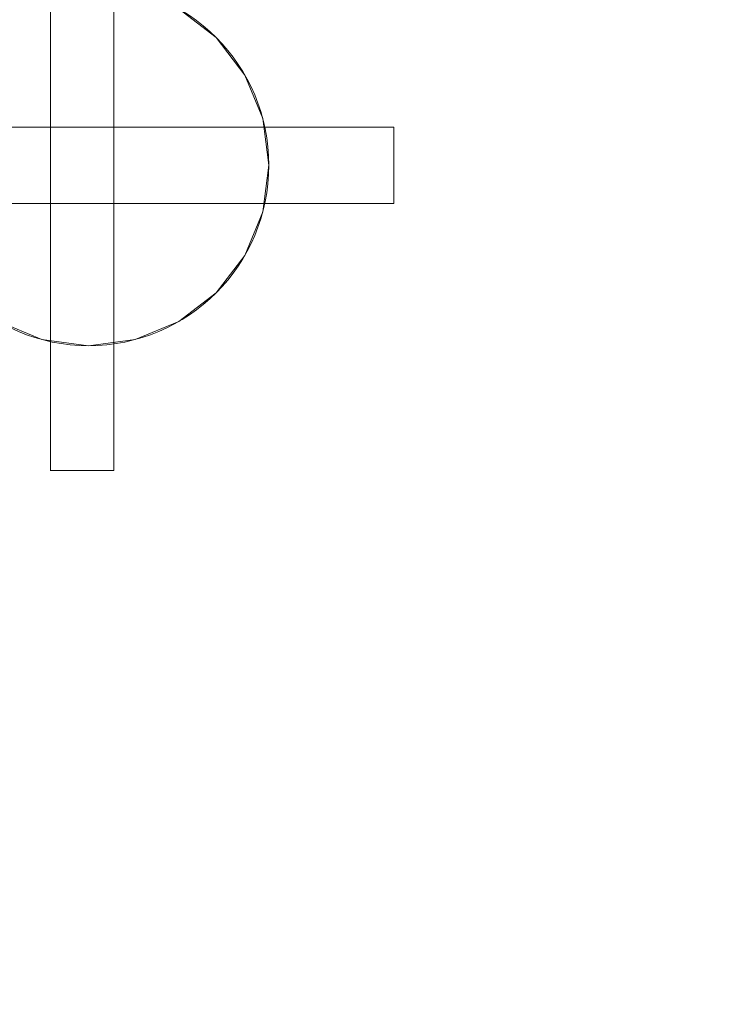
# Model space of a CAD drawing. Units: inches. Extents: x 2696 to 3240, y 1564 to 2310.
# Tile 45 of 76: x 2782.926 to 2786.339, y 2084.368 to 2089.203. Entities that reach past the tile are written whole.
import ezdxf

# ---------------------------------------------------------------- set-up
doc = ezdxf.new("R2010")
doc.units = ezdxf.units.IN
for name, color, linetype, lineweight in [('A-ANNO-DIMS', 3, 'Continuous', 18), ('A-FLOR-FIXT', 8, 'Continuous', 18), ('A-FURN', 251, 'Continuous', 13)]:
    doc.layers.add(name, color=color, linetype=linetype, lineweight=lineweight)
doc.styles.add('TIMES NEW', font='times.ttf')
doc.dimstyles.new('Siddhuu', dxfattribs={"dimtxt": 6, "dimasz": 2.5, "dimexe": 1.25, "dimexo": 0.625, "dimtad": 1, "dimdec": 1, "dimlunit": 4, "dimtxsty": 'TIMES NEW', "dimcen": 2.5, "dimclrd": 256, "dimclre": 1, "dimclrt": 7, "dimadec": 0, "dimazin": 0, "dimtfac": 1, "dimtdec": 1, "dimtmove": 0, "dimatfit": 3, "dimfxl": 1, "dimtolj": 1, "dimlwd": -1, "dimarcsym": 0})

# ---------------------------------------------------------------- blocks, each defined once
blk = doc.blocks.new('A$C1af1f523')
at = {"layer": 'A-FURN'}
for p, q in [((-2.9003, 3.9351), (-2.9003, 0.9365)), ((-2.9003, 3.9351, 0.5), (-2.9003, 0.9365, 0.5)), ((-2.9003, 3.9351), (-2.9003, 3.9351, 0.5)), ((-2.5253, 3.9351), (-2.9003, 3.9351)), ((-2.5253, 3.9351, 0.5), (-2.9003, 3.9351, 0.5)), ((-2.5253, 3.9351), (-2.5253, 0.9365)), ((-2.5253, 3.9351, 0.5), (-2.5253, 0.9365, 0.5)), ((-2.5253, 3.9351), (-2.5253, 3.9351, 0.5)), ((-2.9421, 3.2913), (-2.9421, 3.2913, 0.5)), ((-2.7128, 3.3215), (-2.7128, 3.3215, 0.5)), ((-2.4835, 3.2913), (-2.4835, 3.2913, 0.5)), ((-3.1558, 3.2028), (-3.1558, 3.2028, 0.5)), ((-2.2698, 3.2028), (-2.2698, 3.2028, 0.5)), ((-3.3393, 3.062), (-3.3393, 3.062, 0.5)), ((-2.0863, 3.062), (-2.0863, 3.062, 0.5)), ((-3.4801, 2.8785), (-3.4801, 2.8785, 0.5)), ((-3.5686, 2.6648), (-3.5686, 2.6648, 0.5)), ((0, 2.5605), (-4.2116, 2.5605)), ((0, 2.5605, 0.5), (-4.2116, 2.5605, 0.5)), ((-4.2116, 2.5605), (-4.2116, 2.5605, 0.5)), ((-4.2116, 2.5594), (-4.2116, 2.248)), ((-4.2116, 2.5594, 0.5), (-4.2116, 2.248, 0.5)), ((-4.2116, 2.5594), (-4.2116, 2.5594, 0.5)), ((-3.5988, 2.4355), (-3.5988, 2.4355, 0.5)), ((0, 2.248), (-4.2116, 2.248)), ((0, 2.248, 0.5), (-4.2116, 2.248, 0.5)), ((-4.2116, 2.248), (-4.2116, 2.248, 0.5)), ((-4.2116, 2.248), (-4.2116, 2.2469)), ((-4.2116, 2.248, 0.5), (-4.2116, 2.2469, 0.5)), ((-4.2116, 2.2469), (-4.2116, 2.2469, 0.5)), ((-3.5686, 2.2061), (-3.5686, 2.2061, 0.5))]:
    blk.add_line(p, q, dxfattribs=at)
for centre in [(-2.7128, 2.4355), (-2.7128, 2.4355, 0.5)]:
    blk.add_circle(centre, 0.886, dxfattribs=at)
mesh = blk.add_polyface(dxfattribs=at)
corners = [(-2.9003, 0.9365, 0.5), (-2.9003, 3.9351), (-2.9003, 0.9365), (-2.9003, 3.9351, 0.5)]
mesh.append_faces([[corners[k] for k in face] for face in [(2, 1, 0), (3, 0, 1)]], dxfattribs={"vtx1": -1})
mesh = blk.add_polyface(dxfattribs=at)
corners = [(-2.5253, 3.9351, 0.5), (-2.9003, 3.9351), (-2.9003, 3.9351, 0.5), (-2.5253, 3.9351)]
mesh.append_faces([[corners[k] for k in face] for face in [(2, 1, 0), (3, 0, 1)]], dxfattribs={"vtx1": -1})
mesh = blk.add_polyface(dxfattribs=at)
corners = [(-2.5253, 0.9365, 0.5), (-2.5253, 3.9351), (-2.5253, 0.9365), (-2.5253, 3.9351, 0.5)]
mesh.append_faces([[corners[k] for k in face] for face in [(2, 1, 0), (3, 0, 1)]], dxfattribs={"vtx1": -1})
mesh = blk.add_polyface(dxfattribs=at)
corners = [(-2.9421, 3.2913), (-3.1558, 3.2028, 0.5), (-3.1558, 3.2028), (-2.9421, 3.2913, 0.5)]
mesh.append_faces([[corners[k] for k in face] for face in [(2, 1, 0), (3, 0, 1)]], dxfattribs={"vtx1": -1})
mesh = blk.add_polyface(dxfattribs=at)
corners = [(-2.7128, 3.3215), (-2.9421, 3.2913, 0.5), (-2.9421, 3.2913), (-2.7128, 3.3215, 0.5)]
mesh.append_faces([[corners[k] for k in face] for face in [(2, 1, 0), (3, 0, 1)]], dxfattribs={"vtx1": -1})
mesh = blk.add_polyface(dxfattribs=at)
corners = [(-2.4835, 3.2913), (-2.7128, 3.3215, 0.5), (-2.7128, 3.3215), (-2.4835, 3.2913, 0.5)]
mesh.append_faces([[corners[k] for k in face] for face in [(2, 1, 0), (3, 0, 1)]], dxfattribs={"vtx1": -1})
mesh = blk.add_polyface(dxfattribs=at)
corners = [(-2.2698, 3.2028), (-2.4835, 3.2913, 0.5), (-2.4835, 3.2913), (-2.2698, 3.2028, 0.5)]
mesh.append_faces([[corners[k] for k in face] for face in [(2, 1, 0), (3, 0, 1)]], dxfattribs={"vtx1": -1})
mesh = blk.add_polyface(dxfattribs=at)
corners = [(-3.1558, 3.2028), (-3.3393, 3.062, 0.5), (-3.3393, 3.062), (-3.1558, 3.2028, 0.5)]
mesh.append_faces([[corners[k] for k in face] for face in [(2, 1, 0), (3, 0, 1)]], dxfattribs={"vtx1": -1})
mesh = blk.add_polyface(dxfattribs=at)
corners = [(-2.0863, 3.062), (-2.2698, 3.2028, 0.5), (-2.2698, 3.2028), (-2.0863, 3.062, 0.5)]
mesh.append_faces([[corners[k] for k in face] for face in [(2, 1, 0), (3, 0, 1)]], dxfattribs={"vtx1": -1})
mesh = blk.add_polyface(dxfattribs=at)
corners = [(-3.3393, 3.062, 0.5), (-3.4801, 2.8785), (-3.3393, 3.062), (-3.4801, 2.8785, 0.5)]
mesh.append_faces([[corners[k] for k in face] for face in [(2, 1, 0), (3, 0, 1)]], dxfattribs={"vtx1": -1})
mesh = blk.add_polyface(dxfattribs=at)
corners = [(-1.9455, 2.8785, 0.5), (-2.0863, 3.062), (-1.9455, 2.8785), (-2.0863, 3.062, 0.5)]
mesh.append_faces([[corners[k] for k in face] for face in [(2, 1, 0), (3, 0, 1)]], dxfattribs={"vtx1": -1})
mesh = blk.add_polyface(dxfattribs=at)
corners = [(-3.4801, 2.8785, 0.5), (-3.5686, 2.6648), (-3.4801, 2.8785), (-3.5686, 2.6648, 0.5)]
mesh.append_faces([[corners[k] for k in face] for face in [(2, 1, 0), (3, 0, 1)]], dxfattribs={"vtx1": -1})
mesh = blk.add_polyface(dxfattribs=at)
corners = [(-3.5686, 2.6648, 0.5), (-3.5988, 2.4355), (-3.5686, 2.6648), (-3.5988, 2.4355, 0.5)]
mesh.append_faces([[corners[k] for k in face] for face in [(2, 1, 0), (3, 0, 1)]], dxfattribs={"vtx1": -1})
mesh = blk.add_polyface(dxfattribs=at)
corners = [(0, 2.5605, 0.5), (-4.2116, 2.5605), (-4.2116, 2.5605, 0.5), (0, 2.5605)]
mesh.append_faces([[corners[k] for k in face] for face in [(2, 1, 0), (3, 0, 1)]], dxfattribs={"vtx1": -1})
mesh = blk.add_polyface(dxfattribs=at)
corners = [(-4.2116, 2.2469, 0.5), (-4.2116, 2.248), (-4.2116, 2.2469), (-4.2116, 2.5594), (-4.2116, 2.5594, 0.5), (-4.2116, 2.248, 0.5)]
mesh.append_faces([[corners[k] for k in face] for face in [(3, 0, 1), (4, 0, 3)]], dxfattribs={"vtx0": -1, "vtx1": -1})
mesh.append_faces([[corners[k] for k in face] for face in [(2, 1, 0), (5, 0, 4)]], dxfattribs={"vtx1": -1})
mesh = blk.add_polyface(dxfattribs=at)
corners = [(-3.5988, 2.4355, 0.5), (-3.5686, 2.2061), (-3.5988, 2.4355), (-3.5686, 2.2061, 0.5)]
mesh.append_faces([[corners[k] for k in face] for face in [(2, 1, 0), (3, 0, 1)]], dxfattribs={"vtx1": -1})
mesh = blk.add_polyface(dxfattribs=at)
corners = [(0, 2.248, 0.5), (-4.2116, 2.248), (-4.2116, 2.248, 0.5), (0, 2.248)]
mesh.append_faces([[corners[k] for k in face] for face in [(2, 1, 0), (3, 0, 1)]], dxfattribs={"vtx1": -1})
mesh = blk.add_polyface(dxfattribs=at)
corners = [(-3.5686, 2.2061, 0.5), (-3.4801, 1.9924), (-3.5686, 2.2061), (-3.4801, 1.9924, 0.5)]
mesh.append_faces([[corners[k] for k in face] for face in [(2, 1, 0), (3, 0, 1)]], dxfattribs={"vtx1": -1})
blk = doc.blocks.new('*D40')
at = {"layer": 'A-ANNO-DIMS', "color": 1, "lineweight": -2, "transparency": 16777216}
for p, q in [((2777.2662, 2091.8261), (2777.2662, 2093.5758)), ((2784.7641, 2091.8261), (2784.7641, 2093.5758))]:
    blk.add_line(p, q, dxfattribs=at)
at = {"layer": 'A-ANNO-DIMS', "transparency": 16777216}
for p, q in [((2779.7662, 2092.3258), (2782.2641, 2092.3258)), ((2784.7641, 2092.3258), (2902.4579, 2092.3258))]:
    blk.add_line(p, q, dxfattribs=at)
for points in [[(2779.7662, 2092.7424), (2779.7662, 2091.9091), (2777.2662, 2092.3258)], [(2782.2641, 2092.7424), (2782.2641, 2091.9091), (2784.7641, 2092.3258)]]:
    blk.add_solid(points, dxfattribs=at)
at = {"layer": 'Defpoints', "color": 0, "transparency": 16777216}
for p in [(2784.7641, 2092.3258), (2777.2662, 2091.2011), (2784.7641, 2091.2011)]:
    blk.add_point(p, dxfattribs=at)
at = {"layer": 'A-ANNO-DIMS', "color": 7, "transparency": 16777216, "insert": (2844.861, 2096.0935), "char_height": 6, "attachment_point": 5, "style": 'TIMES NEW'}
blk.add_mtext('\\A1;BATH FITTING 0\'-7 1/2" TYP.', dxfattribs=at)
blk = doc.blocks.new('*D41')
at = {"layer": 'A-ANNO-DIMS', "transparency": 16777216}
for p, q in [((2776.1416, 2091.2011), (2776.1416, 2145.7283)), ((2776.1416, 2087.1996), (2776.1416, 2088.7011))]:
    blk.add_line(p, q, dxfattribs=at)
at = {"layer": 'A-ANNO-DIMS', "color": 1, "lineweight": -2, "transparency": 16777216}
for p, q in [((2776.6412, 2091.2011), (2774.8916, 2091.2011)), ((2776.6412, 2084.6996), (2774.8916, 2084.6996))]:
    blk.add_line(p, q, dxfattribs=at)
at = {"layer": 'A-ANNO-DIMS', "transparency": 16777216}
for points in [[(2775.7249, 2088.7011), (2776.5582, 2088.7011), (2776.1416, 2091.2011)], [(2775.7249, 2087.1996), (2776.5582, 2087.1996), (2776.1416, 2084.6996)]]:
    blk.add_solid(points, dxfattribs=at)
at = {"layer": 'Defpoints', "color": 0, "transparency": 16777216}
for p in [(2776.1416, 2091.2011), (2777.2662, 2091.2011), (2777.2662, 2084.6996)]:
    blk.add_point(p, dxfattribs=at)
at = {"layer": 'A-ANNO-DIMS', "color": 7, "transparency": 16777216, "insert": (2772.3803, 2119.7147), "char_height": 6, "attachment_point": 5, "rotation": 90, "style": 'TIMES NEW'}
blk.add_mtext('\\A1;0\'-6 1/2" TYP.', dxfattribs=at)
blk = doc.blocks.new('*D62')
at = {"layer": 'A-ANNO-DIMS', "color": 1, "lineweight": -2, "transparency": 16777216}
for p, q in [((2965.0838, 2140.7011), (2709.3614, 2140.7011)), ((2965.0838, 2063.5906), (2709.3614, 2063.5906))]:
    blk.add_line(p, q, dxfattribs=at)
at = {"layer": 'A-ANNO-DIMS', "transparency": 16777216}
blk.add_line((2710.6114, 2066.0906), (2710.6114, 2138.2011), dxfattribs=at)
for points in [[(2710.1947, 2138.2011), (2711.0281, 2138.2011), (2710.6114, 2140.7011)], [(2710.1947, 2066.0906), (2711.0281, 2066.0906), (2710.6114, 2063.5906)]]:
    blk.add_solid(points, dxfattribs=at)
at = {"layer": 'Defpoints', "color": 0, "transparency": 16777216}
for p in [(2710.6114, 2140.7011), (2965.7088, 2140.7011), (2965.7088, 2063.5906)]:
    blk.add_point(p, dxfattribs=at)
at = {"layer": 'A-ANNO-DIMS', "color": 7, "transparency": 16777216, "insert": (2706.9345, 2102.1459), "char_height": 6, "attachment_point": 5, "rotation": 90, "style": 'TIMES NEW'}
blk.add_mtext('\\A1;6\'-5"', dxfattribs=at)
blk = doc.blocks.new('*D64')
at = {"layer": 'A-ANNO-DIMS', "color": 1, "lineweight": -2, "transparency": 16777216}
for p, q in [((3073.0838, 2206.7011), (2709.3614, 2206.7011)), ((3068.5838, 1989.2011), (2709.3614, 1989.2011))]:
    blk.add_line(p, q, dxfattribs=at)
at = {"layer": 'A-ANNO-DIMS', "transparency": 16777216}
blk.add_line((2710.6114, 1991.7011), (2710.6114, 2204.2011), dxfattribs=at)
for points in [[(2710.1947, 2204.2011), (2711.0281, 2204.2011), (2710.6114, 2206.7011)], [(2710.1947, 1991.7011), (2711.0281, 1991.7011), (2710.6114, 1989.2011)]]:
    blk.add_solid(points, dxfattribs=at)
at = {"layer": 'Defpoints', "color": 0, "transparency": 16777216}
for p in [(2710.6114, 2206.7011), (3073.7088, 2206.7011), (3069.2088, 1989.2011)]:
    blk.add_point(p, dxfattribs=at)
at = {"layer": 'A-ANNO-DIMS', "color": 7, "transparency": 16777216, "insert": (2706.8501, 2097.9511), "char_height": 6, "attachment_point": 5, "rotation": 90, "style": 'TIMES NEW'}
blk.add_mtext('\\A1;18\'-1 1/2"', dxfattribs=at)
blk = doc.blocks.new('*D66')
at = {"layer": 'A-ANNO-DIMS', "color": 1, "lineweight": -2, "transparency": 16777216}
for p, q in [((3077.5838, 2122.7011), (2709.3614, 2122.7011)), ((3077.5838, 2074.7011), (2709.3614, 2074.7011))]:
    blk.add_line(p, q, dxfattribs=at)
at = {"layer": 'A-ANNO-DIMS', "transparency": 16777216}
blk.add_line((2710.6114, 2077.2011), (2710.6114, 2120.2011), dxfattribs=at)
for points in [[(2710.1947, 2120.2011), (2711.0281, 2120.2011), (2710.6114, 2122.7011)], [(2710.1947, 2077.2011), (2711.0281, 2077.2011), (2710.6114, 2074.7011)]]:
    blk.add_solid(points, dxfattribs=at)
at = {"layer": 'Defpoints', "color": 0, "transparency": 16777216}
for p in [(2710.6114, 2122.7011), (3078.2088, 2122.7011), (3078.2088, 2074.7011)]:
    blk.add_point(p, dxfattribs=at)
at = {"layer": 'A-ANNO-DIMS', "color": 7, "transparency": 16777216, "insert": (2706.9345, 2098.7011), "char_height": 6, "attachment_point": 5, "rotation": 90, "style": 'TIMES NEW'}
blk.add_mtext('\\A1;4\'-0"', dxfattribs=at)

msp = doc.modelspace()

# ---------------------------------------------------------------- block references
at = {"layer": 'A-FLOR-FIXT', "xscale": -1, "rotation": 270}
msp.add_blockref('A$C1af1f523', (2780.829, 2091.2011), dxfattribs=at)

# ---------------------------------------------------------------- dimensions: what is measured, and where the dimension line sits
at = {"layer": 'A-ANNO-DIMS'}
for base, p1, p2, picture, middle in [((2710.6114, 2206.7011), (3069.2088, 1989.2011), (3073.7088, 2206.7011), '*D64', (2706.8501, 2097.9511)), ((2710.6114, 2140.7011), (2965.7088, 2063.5906), (2965.7088, 2140.7011), '*D62', (2706.9345, 2102.1459)), ((2710.6114, 2122.7011), (3078.2088, 2074.7011), (3078.2088, 2122.7011), '*D66', (2706.9345, 2098.7011))]:
    dim = msp.add_linear_dim(base=base, p1=p1, p2=p2, angle=90, dimstyle='Siddhuu', override={"dimdec": 1, "dimlfac": 1, "dimrnd": 0, "dimzin": 1, "dimdsep": 46, "dimlunit": 4, "dimfrac": 2}, dxfattribs=at)
    dim.commit()
    dim.dimension.update_dxf_attribs({"geometry": picture, "text_midpoint": middle})
dim = msp.add_linear_dim(base=(2776.1416, 2091.2011), p1=(2777.2662, 2084.6996), p2=(2777.2662, 2091.2011), angle=90, text='<> TYP.', dimstyle='Siddhuu', override={"dimdec": 1, "dimlfac": 1, "dimrnd": 0, "dimzin": 1, "dimdsep": 46, "dimlunit": 4, "dimfrac": 2}, dxfattribs=at)
dim.commit()
dim.dimension.update_dxf_attribs({"geometry": '*D41', "text_midpoint": (2772.3803, 2119.7147)})
dim = msp.add_linear_dim(base=(2784.7641, 2092.3258), p1=(2777.2662, 2091.2011), p2=(2784.7641, 2091.2011), text='BATH FITTING <> TYP.', dimstyle='Siddhuu', override={"dimdec": 1, "dimlfac": 1, "dimrnd": 0, "dimzin": 1, "dimdsep": 46, "dimlunit": 4, "dimfrac": 2}, dxfattribs=at)
dim.commit()
dim.dimension.update_dxf_attribs({"geometry": '*D40', "text_midpoint": (2844.861, 2096.0935)})

doc.saveas('drawing.dxf')
